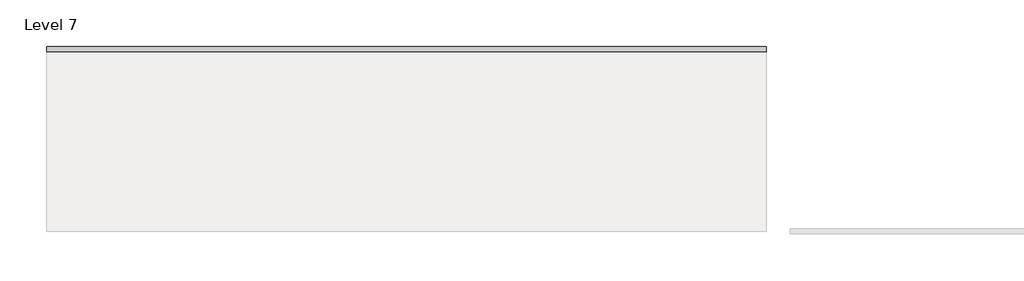
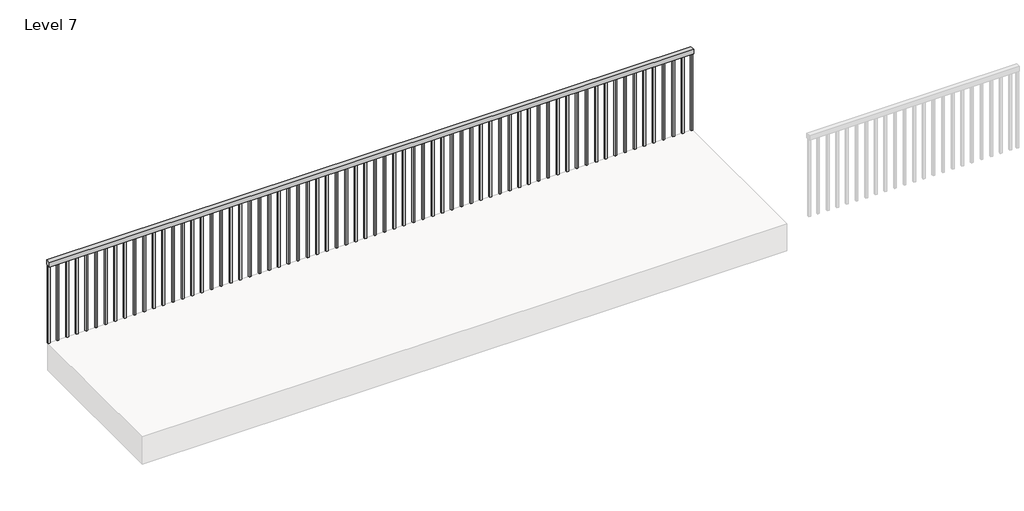
# One storey, part 5 of 5: 1 railing.
"""IFC4 building model written with IfcOpenShell, lengths in millimetres."""

from ifc_helpers import new_model, si_unit, frame, origin, place, context, project, spatial, polyline, outline, extrude, element, save

model = new_model("IFC4")

# Units and contexts
model_context = context("Model", 3, world=origin())
ifc_project = project(units=[si_unit("LENGTHUNIT", "METRE", prefix="MILLI")], contexts=[model_context])

# Site, building, storey
site = spatial("IfcSite", under=ifc_project)
building = spatial("IfcBuilding", under=site)
storey = spatial("IfcBuildingStorey", under=building, Name="Level 7", Elevation=6400.8)

# Railing
placement = place(None, origin())
element("IfcRailing", 1, ObjectType="Handrail - Rectangular", at=placement, inside=storey, context=model_context, shape_type="SweptSolid", body=[
    extrude(outline(polyline([(7096.1361222, 16470.4237525), (7096.1361222, 16521.2237525), (13903.3361222, 16521.2237525), (13903.3361222, 16470.4237525), (7096.1361222, 16470.4237525)])), frame((0.0, 0.0, 7264.4), z_axis=(0.0, 0.0, 1.0), x_axis=(1.0, 0.0, 0.0)), (0.0, 0.0, 1.0), 50.8),
    extrude(outline(polyline([(13792.2111222, 16486.2987525), (13792.2111222, 16505.3487525), (13811.2611222, 16505.3487525), (13811.2611222, 16486.2987525), (13792.2111222, 16486.2987525)])), frame((0.0, 0.0, 6400.8), z_axis=(0.0, 0.0, 1.0), x_axis=(1.0, 0.0, 0.0)), (0.0, 0.0, 1.0), 863.6),
    extrude(outline(polyline([(13690.6111222, 16486.2987525), (13690.6111222, 16505.3487525), (13709.6611222, 16505.3487525), (13709.6611222, 16486.2987525), (13690.6111222, 16486.2987525)])), frame((0.0, 0.0, 6400.8), z_axis=(0.0, 0.0, 1.0), x_axis=(1.0, 0.0, 0.0)), (0.0, 0.0, 1.0), 863.6),
    extrude(outline(polyline([(13589.0111222, 16486.2987525), (13589.0111222, 16505.3487525), (13608.0611222, 16505.3487525), (13608.0611222, 16486.2987525), (13589.0111222, 16486.2987525)])), frame((0.0, 0.0, 6400.8), z_axis=(0.0, 0.0, 1.0), x_axis=(1.0, 0.0, 0.0)), (0.0, 0.0, 1.0), 863.6),
    extrude(outline(polyline([(13487.4111222, 16486.2987525), (13487.4111222, 16505.3487525), (13506.4611222, 16505.3487525), (13506.4611222, 16486.2987525), (13487.4111222, 16486.2987525)])), frame((0.0, 0.0, 6400.8), z_axis=(0.0, 0.0, 1.0), x_axis=(1.0, 0.0, 0.0)), (0.0, 0.0, 1.0), 863.6),
    extrude(outline(polyline([(13385.8111222, 16486.2987525), (13385.8111222, 16505.3487525), (13404.8611222, 16505.3487525), (13404.8611222, 16486.2987525), (13385.8111222, 16486.2987525)])), frame((0.0, 0.0, 6400.8), z_axis=(0.0, 0.0, 1.0), x_axis=(1.0, 0.0, 0.0)), (0.0, 0.0, 1.0), 863.6),
    extrude(outline(polyline([(13284.2111222, 16486.2987525), (13284.2111222, 16505.3487525), (13303.2611222, 16505.3487525), (13303.2611222, 16486.2987525), (13284.2111222, 16486.2987525)])), frame((0.0, 0.0, 6400.8), z_axis=(0.0, 0.0, 1.0), x_axis=(1.0, 0.0, 0.0)), (0.0, 0.0, 1.0), 863.6),
    extrude(outline(polyline([(13182.6111222, 16486.2987525), (13182.6111222, 16505.3487525), (13201.6611222, 16505.3487525), (13201.6611222, 16486.2987525), (13182.6111222, 16486.2987525)])), frame((0.0, 0.0, 6400.8), z_axis=(0.0, 0.0, 1.0), x_axis=(1.0, 0.0, 0.0)), (0.0, 0.0, 1.0), 863.6),
    extrude(outline(polyline([(13081.0111222, 16486.2987525), (13081.0111222, 16505.3487525), (13100.0611222, 16505.3487525), (13100.0611222, 16486.2987525), (13081.0111222, 16486.2987525)])), frame((0.0, 0.0, 6400.8), z_axis=(0.0, 0.0, 1.0), x_axis=(1.0, 0.0, 0.0)), (0.0, 0.0, 1.0), 863.6),
    extrude(outline(polyline([(12979.4111222, 16486.2987525), (12979.4111222, 16505.3487525), (12998.4611222, 16505.3487525), (12998.4611222, 16486.2987525), (12979.4111222, 16486.2987525)])), frame((0.0, 0.0, 6400.8), z_axis=(0.0, 0.0, 1.0), x_axis=(1.0, 0.0, 0.0)), (0.0, 0.0, 1.0), 863.6),
    extrude(outline(polyline([(12877.8111222, 16486.2987525), (12877.8111222, 16505.3487525), (12896.8611222, 16505.3487525), (12896.8611222, 16486.2987525), (12877.8111222, 16486.2987525)])), frame((0.0, 0.0, 6400.8), z_axis=(0.0, 0.0, 1.0), x_axis=(1.0, 0.0, 0.0)), (0.0, 0.0, 1.0), 863.6),
    extrude(outline(polyline([(12776.2111222, 16486.2987525), (12776.2111222, 16505.3487525), (12795.2611222, 16505.3487525), (12795.2611222, 16486.2987525), (12776.2111222, 16486.2987525)])), frame((0.0, 0.0, 6400.8), z_axis=(0.0, 0.0, 1.0), x_axis=(1.0, 0.0, 0.0)), (0.0, 0.0, 1.0), 863.6),
    extrude(outline(polyline([(12674.6111222, 16486.2987525), (12674.6111222, 16505.3487525), (12693.6611222, 16505.3487525), (12693.6611222, 16486.2987525), (12674.6111222, 16486.2987525)])), frame((0.0, 0.0, 6400.8), z_axis=(0.0, 0.0, 1.0), x_axis=(1.0, 0.0, 0.0)), (0.0, 0.0, 1.0), 863.6),
    extrude(outline(polyline([(12573.0111222, 16486.2987525), (12573.0111222, 16505.3487525), (12592.0611222, 16505.3487525), (12592.0611222, 16486.2987525), (12573.0111222, 16486.2987525)])), frame((0.0, 0.0, 6400.8), z_axis=(0.0, 0.0, 1.0), x_axis=(1.0, 0.0, 0.0)), (0.0, 0.0, 1.0), 863.6),
    extrude(outline(polyline([(12471.4111222, 16486.2987525), (12471.4111222, 16505.3487525), (12490.4611222, 16505.3487525), (12490.4611222, 16486.2987525), (12471.4111222, 16486.2987525)])), frame((0.0, 0.0, 6400.8), z_axis=(0.0, 0.0, 1.0), x_axis=(1.0, 0.0, 0.0)), (0.0, 0.0, 1.0), 863.6),
    extrude(outline(polyline([(12369.8111222, 16486.2987525), (12369.8111222, 16505.3487525), (12388.8611222, 16505.3487525), (12388.8611222, 16486.2987525), (12369.8111222, 16486.2987525)])), frame((0.0, 0.0, 6400.8), z_axis=(0.0, 0.0, 1.0), x_axis=(1.0, 0.0, 0.0)), (0.0, 0.0, 1.0), 863.6),
    extrude(outline(polyline([(12268.2111222, 16486.2987525), (12268.2111222, 16505.3487525), (12287.2611222, 16505.3487525), (12287.2611222, 16486.2987525), (12268.2111222, 16486.2987525)])), frame((0.0, 0.0, 6400.8), z_axis=(0.0, 0.0, 1.0), x_axis=(1.0, 0.0, 0.0)), (0.0, 0.0, 1.0), 863.6),
    extrude(outline(polyline([(12166.6111222, 16486.2987525), (12166.6111222, 16505.3487525), (12185.6611222, 16505.3487525), (12185.6611222, 16486.2987525), (12166.6111222, 16486.2987525)])), frame((0.0, 0.0, 6400.8), z_axis=(0.0, 0.0, 1.0), x_axis=(1.0, 0.0, 0.0)), (0.0, 0.0, 1.0), 863.6),
    extrude(outline(polyline([(12065.0111222, 16486.2987525), (12065.0111222, 16505.3487525), (12084.0611222, 16505.3487525), (12084.0611222, 16486.2987525), (12065.0111222, 16486.2987525)])), frame((0.0, 0.0, 6400.8), z_axis=(0.0, 0.0, 1.0), x_axis=(1.0, 0.0, 0.0)), (0.0, 0.0, 1.0), 863.6),
    extrude(outline(polyline([(11963.4111222, 16486.2987525), (11963.4111222, 16505.3487525), (11982.4611222, 16505.3487525), (11982.4611222, 16486.2987525), (11963.4111222, 16486.2987525)])), frame((0.0, 0.0, 6400.8), z_axis=(0.0, 0.0, 1.0), x_axis=(1.0, 0.0, 0.0)), (0.0, 0.0, 1.0), 863.6),
    extrude(outline(polyline([(11861.8111222, 16486.2987525), (11861.8111222, 16505.3487525), (11880.8611222, 16505.3487525), (11880.8611222, 16486.2987525), (11861.8111222, 16486.2987525)])), frame((0.0, 0.0, 6400.8), z_axis=(0.0, 0.0, 1.0), x_axis=(1.0, 0.0, 0.0)), (0.0, 0.0, 1.0), 863.6),
    extrude(outline(polyline([(11760.2111222, 16486.2987525), (11760.2111222, 16505.3487525), (11779.2611222, 16505.3487525), (11779.2611222, 16486.2987525), (11760.2111222, 16486.2987525)])), frame((0.0, 0.0, 6400.8), z_axis=(0.0, 0.0, 1.0), x_axis=(1.0, 0.0, 0.0)), (0.0, 0.0, 1.0), 863.6),
    extrude(outline(polyline([(11658.6111222, 16486.2987525), (11658.6111222, 16505.3487525), (11677.6611222, 16505.3487525), (11677.6611222, 16486.2987525), (11658.6111222, 16486.2987525)])), frame((0.0, 0.0, 6400.8), z_axis=(0.0, 0.0, 1.0), x_axis=(1.0, 0.0, 0.0)), (0.0, 0.0, 1.0), 863.6),
    extrude(outline(polyline([(11557.0111222, 16486.2987525), (11557.0111222, 16505.3487525), (11576.0611222, 16505.3487525), (11576.0611222, 16486.2987525), (11557.0111222, 16486.2987525)])), frame((0.0, 0.0, 6400.8), z_axis=(0.0, 0.0, 1.0), x_axis=(1.0, 0.0, 0.0)), (0.0, 0.0, 1.0), 863.6),
    extrude(outline(polyline([(11455.4111222, 16486.2987525), (11455.4111222, 16505.3487525), (11474.4611222, 16505.3487525), (11474.4611222, 16486.2987525), (11455.4111222, 16486.2987525)])), frame((0.0, 0.0, 6400.8), z_axis=(0.0, 0.0, 1.0), x_axis=(1.0, 0.0, 0.0)), (0.0, 0.0, 1.0), 863.6),
    extrude(outline(polyline([(11353.8111222, 16486.2987525), (11353.8111222, 16505.3487525), (11372.8611222, 16505.3487525), (11372.8611222, 16486.2987525), (11353.8111222, 16486.2987525)])), frame((0.0, 0.0, 6400.8), z_axis=(0.0, 0.0, 1.0), x_axis=(1.0, 0.0, 0.0)), (0.0, 0.0, 1.0), 863.6),
    extrude(outline(polyline([(11252.2111222, 16486.2987525), (11252.2111222, 16505.3487525), (11271.2611222, 16505.3487525), (11271.2611222, 16486.2987525), (11252.2111222, 16486.2987525)])), frame((0.0, 0.0, 6400.8), z_axis=(0.0, 0.0, 1.0), x_axis=(1.0, 0.0, 0.0)), (0.0, 0.0, 1.0), 863.6),
    extrude(outline(polyline([(11150.6111222, 16486.2987525), (11150.6111222, 16505.3487525), (11169.6611222, 16505.3487525), (11169.6611222, 16486.2987525), (11150.6111222, 16486.2987525)])), frame((0.0, 0.0, 6400.8), z_axis=(0.0, 0.0, 1.0), x_axis=(1.0, 0.0, 0.0)), (0.0, 0.0, 1.0), 863.6),
    extrude(outline(polyline([(11049.0111222, 16486.2987525), (11049.0111222, 16505.3487525), (11068.0611222, 16505.3487525), (11068.0611222, 16486.2987525), (11049.0111222, 16486.2987525)])), frame((0.0, 0.0, 6400.8), z_axis=(0.0, 0.0, 1.0), x_axis=(1.0, 0.0, 0.0)), (0.0, 0.0, 1.0), 863.6),
    extrude(outline(polyline([(10947.4111222, 16486.2987525), (10947.4111222, 16505.3487525), (10966.4611222, 16505.3487525), (10966.4611222, 16486.2987525), (10947.4111222, 16486.2987525)])), frame((0.0, 0.0, 6400.8), z_axis=(0.0, 0.0, 1.0), x_axis=(1.0, 0.0, 0.0)), (0.0, 0.0, 1.0), 863.6),
    extrude(outline(polyline([(10845.8111222, 16486.2987525), (10845.8111222, 16505.3487525), (10864.8611222, 16505.3487525), (10864.8611222, 16486.2987525), (10845.8111222, 16486.2987525)])), frame((0.0, 0.0, 6400.8), z_axis=(0.0, 0.0, 1.0), x_axis=(1.0, 0.0, 0.0)), (0.0, 0.0, 1.0), 863.6),
    extrude(outline(polyline([(10744.2111222, 16486.2987525), (10744.2111222, 16505.3487525), (10763.2611222, 16505.3487525), (10763.2611222, 16486.2987525), (10744.2111222, 16486.2987525)])), frame((0.0, 0.0, 6400.8), z_axis=(0.0, 0.0, 1.0), x_axis=(1.0, 0.0, 0.0)), (0.0, 0.0, 1.0), 863.6),
    extrude(outline(polyline([(10642.6111222, 16486.2987525), (10642.6111222, 16505.3487525), (10661.6611222, 16505.3487525), (10661.6611222, 16486.2987525), (10642.6111222, 16486.2987525)])), frame((0.0, 0.0, 6400.8), z_axis=(0.0, 0.0, 1.0), x_axis=(1.0, 0.0, 0.0)), (0.0, 0.0, 1.0), 863.6),
    extrude(outline(polyline([(10541.0111222, 16486.2987525), (10541.0111222, 16505.3487525), (10560.0611222, 16505.3487525), (10560.0611222, 16486.2987525), (10541.0111222, 16486.2987525)])), frame((0.0, 0.0, 6400.8), z_axis=(0.0, 0.0, 1.0), x_axis=(1.0, 0.0, 0.0)), (0.0, 0.0, 1.0), 863.6),
    extrude(outline(polyline([(10439.4111222, 16486.2987525), (10439.4111222, 16505.3487525), (10458.4611222, 16505.3487525), (10458.4611222, 16486.2987525), (10439.4111222, 16486.2987525)])), frame((0.0, 0.0, 6400.8), z_axis=(0.0, 0.0, 1.0), x_axis=(1.0, 0.0, 0.0)), (0.0, 0.0, 1.0), 863.6),
    extrude(outline(polyline([(10337.8111222, 16486.2987525), (10337.8111222, 16505.3487525), (10356.8611222, 16505.3487525), (10356.8611222, 16486.2987525), (10337.8111222, 16486.2987525)])), frame((0.0, 0.0, 6400.8), z_axis=(0.0, 0.0, 1.0), x_axis=(1.0, 0.0, 0.0)), (0.0, 0.0, 1.0), 863.6),
    extrude(outline(polyline([(10236.2111222, 16486.2987525), (10236.2111222, 16505.3487525), (10255.2611222, 16505.3487525), (10255.2611222, 16486.2987525), (10236.2111222, 16486.2987525)])), frame((0.0, 0.0, 6400.8), z_axis=(0.0, 0.0, 1.0), x_axis=(1.0, 0.0, 0.0)), (0.0, 0.0, 1.0), 863.6),
    extrude(outline(polyline([(10134.6111222, 16486.2987525), (10134.6111222, 16505.3487525), (10153.6611222, 16505.3487525), (10153.6611222, 16486.2987525), (10134.6111222, 16486.2987525)])), frame((0.0, 0.0, 6400.8), z_axis=(0.0, 0.0, 1.0), x_axis=(1.0, 0.0, 0.0)), (0.0, 0.0, 1.0), 863.6),
    extrude(outline(polyline([(10033.0111222, 16486.2987525), (10033.0111222, 16505.3487525), (10052.0611222, 16505.3487525), (10052.0611222, 16486.2987525), (10033.0111222, 16486.2987525)])), frame((0.0, 0.0, 6400.8), z_axis=(0.0, 0.0, 1.0), x_axis=(1.0, 0.0, 0.0)), (0.0, 0.0, 1.0), 863.6),
    extrude(outline(polyline([(9931.4111222, 16486.2987525), (9931.4111222, 16505.3487525), (9950.4611222, 16505.3487525), (9950.4611222, 16486.2987525), (9931.4111222, 16486.2987525)])), frame((0.0, 0.0, 6400.8), z_axis=(0.0, 0.0, 1.0), x_axis=(1.0, 0.0, 0.0)), (0.0, 0.0, 1.0), 863.6),
    extrude(outline(polyline([(9829.8111222, 16486.2987525), (9829.8111222, 16505.3487525), (9848.8611222, 16505.3487525), (9848.8611222, 16486.2987525), (9829.8111222, 16486.2987525)])), frame((0.0, 0.0, 6400.8), z_axis=(0.0, 0.0, 1.0), x_axis=(1.0, 0.0, 0.0)), (0.0, 0.0, 1.0), 863.6),
    extrude(outline(polyline([(9728.2111222, 16486.2987525), (9728.2111222, 16505.3487525), (9747.2611222, 16505.3487525), (9747.2611222, 16486.2987525), (9728.2111222, 16486.2987525)])), frame((0.0, 0.0, 6400.8), z_axis=(0.0, 0.0, 1.0), x_axis=(1.0, 0.0, 0.0)), (0.0, 0.0, 1.0), 863.6),
    extrude(outline(polyline([(9626.6111222, 16486.2987525), (9626.6111222, 16505.3487525), (9645.6611222, 16505.3487525), (9645.6611222, 16486.2987525), (9626.6111222, 16486.2987525)])), frame((0.0, 0.0, 6400.8), z_axis=(0.0, 0.0, 1.0), x_axis=(1.0, 0.0, 0.0)), (0.0, 0.0, 1.0), 863.6),
    extrude(outline(polyline([(9525.0111222, 16486.2987525), (9525.0111222, 16505.3487525), (9544.0611222, 16505.3487525), (9544.0611222, 16486.2987525), (9525.0111222, 16486.2987525)])), frame((0.0, 0.0, 6400.8), z_axis=(0.0, 0.0, 1.0), x_axis=(1.0, 0.0, 0.0)), (0.0, 0.0, 1.0), 863.6),
    extrude(outline(polyline([(9423.4111222, 16486.2987525), (9423.4111222, 16505.3487525), (9442.4611222, 16505.3487525), (9442.4611222, 16486.2987525), (9423.4111222, 16486.2987525)])), frame((0.0, 0.0, 6400.8), z_axis=(0.0, 0.0, 1.0), x_axis=(1.0, 0.0, 0.0)), (0.0, 0.0, 1.0), 863.6),
    extrude(outline(polyline([(9321.8111222, 16486.2987525), (9321.8111222, 16505.3487525), (9340.8611222, 16505.3487525), (9340.8611222, 16486.2987525), (9321.8111222, 16486.2987525)])), frame((0.0, 0.0, 6400.8), z_axis=(0.0, 0.0, 1.0), x_axis=(1.0, 0.0, 0.0)), (0.0, 0.0, 1.0), 863.6),
    extrude(outline(polyline([(9220.2111222, 16486.2987525), (9220.2111222, 16505.3487525), (9239.2611222, 16505.3487525), (9239.2611222, 16486.2987525), (9220.2111222, 16486.2987525)])), frame((0.0, 0.0, 6400.8), z_axis=(0.0, 0.0, 1.0), x_axis=(1.0, 0.0, 0.0)), (0.0, 0.0, 1.0), 863.6),
    extrude(outline(polyline([(9118.6111222, 16486.2987525), (9118.6111222, 16505.3487525), (9137.6611222, 16505.3487525), (9137.6611222, 16486.2987525), (9118.6111222, 16486.2987525)])), frame((0.0, 0.0, 6400.8), z_axis=(0.0, 0.0, 1.0), x_axis=(1.0, 0.0, 0.0)), (0.0, 0.0, 1.0), 863.6),
    extrude(outline(polyline([(9017.0111222, 16486.2987525), (9017.0111222, 16505.3487525), (9036.0611222, 16505.3487525), (9036.0611222, 16486.2987525), (9017.0111222, 16486.2987525)])), frame((0.0, 0.0, 6400.8), z_axis=(0.0, 0.0, 1.0), x_axis=(1.0, 0.0, 0.0)), (0.0, 0.0, 1.0), 863.6),
    extrude(outline(polyline([(8915.4111222, 16486.2987525), (8915.4111222, 16505.3487525), (8934.4611222, 16505.3487525), (8934.4611222, 16486.2987525), (8915.4111222, 16486.2987525)])), frame((0.0, 0.0, 6400.8), z_axis=(0.0, 0.0, 1.0), x_axis=(1.0, 0.0, 0.0)), (0.0, 0.0, 1.0), 863.6),
    extrude(outline(polyline([(8813.8111222, 16486.2987525), (8813.8111222, 16505.3487525), (8832.8611222, 16505.3487525), (8832.8611222, 16486.2987525), (8813.8111222, 16486.2987525)])), frame((0.0, 0.0, 6400.8), z_axis=(0.0, 0.0, 1.0), x_axis=(1.0, 0.0, 0.0)), (0.0, 0.0, 1.0), 863.6),
    extrude(outline(polyline([(8712.2111222, 16486.2987525), (8712.2111222, 16505.3487525), (8731.2611222, 16505.3487525), (8731.2611222, 16486.2987525), (8712.2111222, 16486.2987525)])), frame((0.0, 0.0, 6400.8), z_axis=(0.0, 0.0, 1.0), x_axis=(1.0, 0.0, 0.0)), (0.0, 0.0, 1.0), 863.6),
    extrude(outline(polyline([(8610.6111222, 16486.2987525), (8610.6111222, 16505.3487525), (8629.6611222, 16505.3487525), (8629.6611222, 16486.2987525), (8610.6111222, 16486.2987525)])), frame((0.0, 0.0, 6400.8), z_axis=(0.0, 0.0, 1.0), x_axis=(1.0, 0.0, 0.0)), (0.0, 0.0, 1.0), 863.6),
    extrude(outline(polyline([(8509.0111222, 16486.2987525), (8509.0111222, 16505.3487525), (8528.0611222, 16505.3487525), (8528.0611222, 16486.2987525), (8509.0111222, 16486.2987525)])), frame((0.0, 0.0, 6400.8), z_axis=(0.0, 0.0, 1.0), x_axis=(1.0, 0.0, 0.0)), (0.0, 0.0, 1.0), 863.6),
    extrude(outline(polyline([(8407.4111222, 16486.2987525), (8407.4111222, 16505.3487525), (8426.4611222, 16505.3487525), (8426.4611222, 16486.2987525), (8407.4111222, 16486.2987525)])), frame((0.0, 0.0, 6400.8), z_axis=(0.0, 0.0, 1.0), x_axis=(1.0, 0.0, 0.0)), (0.0, 0.0, 1.0), 863.6),
    extrude(outline(polyline([(8305.8111222, 16486.2987525), (8305.8111222, 16505.3487525), (8324.8611222, 16505.3487525), (8324.8611222, 16486.2987525), (8305.8111222, 16486.2987525)])), frame((0.0, 0.0, 6400.8), z_axis=(0.0, 0.0, 1.0), x_axis=(1.0, 0.0, 0.0)), (0.0, 0.0, 1.0), 863.6),
    extrude(outline(polyline([(8204.2111222, 16486.2987525), (8204.2111222, 16505.3487525), (8223.2611222, 16505.3487525), (8223.2611222, 16486.2987525), (8204.2111222, 16486.2987525)])), frame((0.0, 0.0, 6400.8), z_axis=(0.0, 0.0, 1.0), x_axis=(1.0, 0.0, 0.0)), (0.0, 0.0, 1.0), 863.6),
    extrude(outline(polyline([(8102.6111222, 16486.2987525), (8102.6111222, 16505.3487525), (8121.6611222, 16505.3487525), (8121.6611222, 16486.2987525), (8102.6111222, 16486.2987525)])), frame((0.0, 0.0, 6400.8), z_axis=(0.0, 0.0, 1.0), x_axis=(1.0, 0.0, 0.0)), (0.0, 0.0, 1.0), 863.6),
    extrude(outline(polyline([(8001.0111222, 16486.2987525), (8001.0111222, 16505.3487525), (8020.0611222, 16505.3487525), (8020.0611222, 16486.2987525), (8001.0111222, 16486.2987525)])), frame((0.0, 0.0, 6400.8), z_axis=(0.0, 0.0, 1.0), x_axis=(1.0, 0.0, 0.0)), (0.0, 0.0, 1.0), 863.6),
    extrude(outline(polyline([(7899.4111222, 16486.2987525), (7899.4111222, 16505.3487525), (7918.4611222, 16505.3487525), (7918.4611222, 16486.2987525), (7899.4111222, 16486.2987525)])), frame((0.0, 0.0, 6400.8), z_axis=(0.0, 0.0, 1.0), x_axis=(1.0, 0.0, 0.0)), (0.0, 0.0, 1.0), 863.6),
    extrude(outline(polyline([(7797.8111222, 16486.2987525), (7797.8111222, 16505.3487525), (7816.8611222, 16505.3487525), (7816.8611222, 16486.2987525), (7797.8111222, 16486.2987525)])), frame((0.0, 0.0, 6400.8), z_axis=(0.0, 0.0, 1.0), x_axis=(1.0, 0.0, 0.0)), (0.0, 0.0, 1.0), 863.6),
    extrude(outline(polyline([(7696.2111222, 16486.2987525), (7696.2111222, 16505.3487525), (7715.2611222, 16505.3487525), (7715.2611222, 16486.2987525), (7696.2111222, 16486.2987525)])), frame((0.0, 0.0, 6400.8), z_axis=(0.0, 0.0, 1.0), x_axis=(1.0, 0.0, 0.0)), (0.0, 0.0, 1.0), 863.6),
    extrude(outline(polyline([(7594.6111222, 16486.2987525), (7594.6111222, 16505.3487525), (7613.6611222, 16505.3487525), (7613.6611222, 16486.2987525), (7594.6111222, 16486.2987525)])), frame((0.0, 0.0, 6400.8), z_axis=(0.0, 0.0, 1.0), x_axis=(1.0, 0.0, 0.0)), (0.0, 0.0, 1.0), 863.6),
    extrude(outline(polyline([(7493.0111222, 16486.2987525), (7493.0111222, 16505.3487525), (7512.0611222, 16505.3487525), (7512.0611222, 16486.2987525), (7493.0111222, 16486.2987525)])), frame((0.0, 0.0, 6400.8), z_axis=(0.0, 0.0, 1.0), x_axis=(1.0, 0.0, 0.0)), (0.0, 0.0, 1.0), 863.6),
    extrude(outline(polyline([(7391.4111222, 16486.2987525), (7391.4111222, 16505.3487525), (7410.4611222, 16505.3487525), (7410.4611222, 16486.2987525), (7391.4111222, 16486.2987525)])), frame((0.0, 0.0, 6400.8), z_axis=(0.0, 0.0, 1.0), x_axis=(1.0, 0.0, 0.0)), (0.0, 0.0, 1.0), 863.6),
    extrude(outline(polyline([(7289.8111222, 16486.2987525), (7289.8111222, 16505.3487525), (7308.8611222, 16505.3487525), (7308.8611222, 16486.2987525), (7289.8111222, 16486.2987525)])), frame((0.0, 0.0, 6400.8), z_axis=(0.0, 0.0, 1.0), x_axis=(1.0, 0.0, 0.0)), (0.0, 0.0, 1.0), 863.6),
    extrude(outline(polyline([(7188.2111222, 16486.2987525), (7188.2111222, 16505.3487525), (7207.2611222, 16505.3487525), (7207.2611222, 16486.2987525), (7188.2111222, 16486.2987525)])), frame((0.0, 0.0, 6400.8), z_axis=(0.0, 0.0, 1.0), x_axis=(1.0, 0.0, 0.0)), (0.0, 0.0, 1.0), 863.6),
    extrude(outline(polyline([(13884.2861222, 16486.2987525), (13884.2861222, 16505.3487525), (13903.3361222, 16505.3487525), (13903.3361222, 16486.2987525), (13884.2861222, 16486.2987525)])), frame((0.0, 0.0, 6400.8), z_axis=(0.0, 0.0, 1.0), x_axis=(1.0, 0.0, 0.0)), (0.0, 0.0, 1.0), 863.6),
    extrude(outline(polyline([(7096.1361222, 16486.2987525), (7096.1361222, 16505.3487525), (7115.1861222, 16505.3487525), (7115.1861222, 16486.2987525), (7096.1361222, 16486.2987525)])), frame((0.0, 0.0, 6400.8), z_axis=(0.0, 0.0, 1.0), x_axis=(1.0, 0.0, 0.0)), (0.0, 0.0, 1.0), 863.6),
])

save(model, "model.ifc")

# Revit data of these elements
# Type "Handrail - Rectangular"
#   Assembly Code = "C2010400"
#   built-in parameter 1008612 = 0.0416667 (stored number, unit not read)
#   built-in parameter 1008611 = 0.0416667 (stored number, unit not read)
#   built-in parameter 1008609 = 0.333333 (stored number, unit not read)
#   built-in parameter 1008604 = 0.166667 (stored number, unit not read)
#   built-in parameter 1008603 = 0.166667 (stored number, unit not read)
#   Railing Height = 3' - 0"
#   built-in parameter 1008630 = 2
#   built-in parameter 1008610 = 2
#   built-in parameter 1008618 = Baluster - Square : 3/4"
# Element 1 (IfcRailing, "Handrail - Rectangular")
#   Phase Created = New Construction
